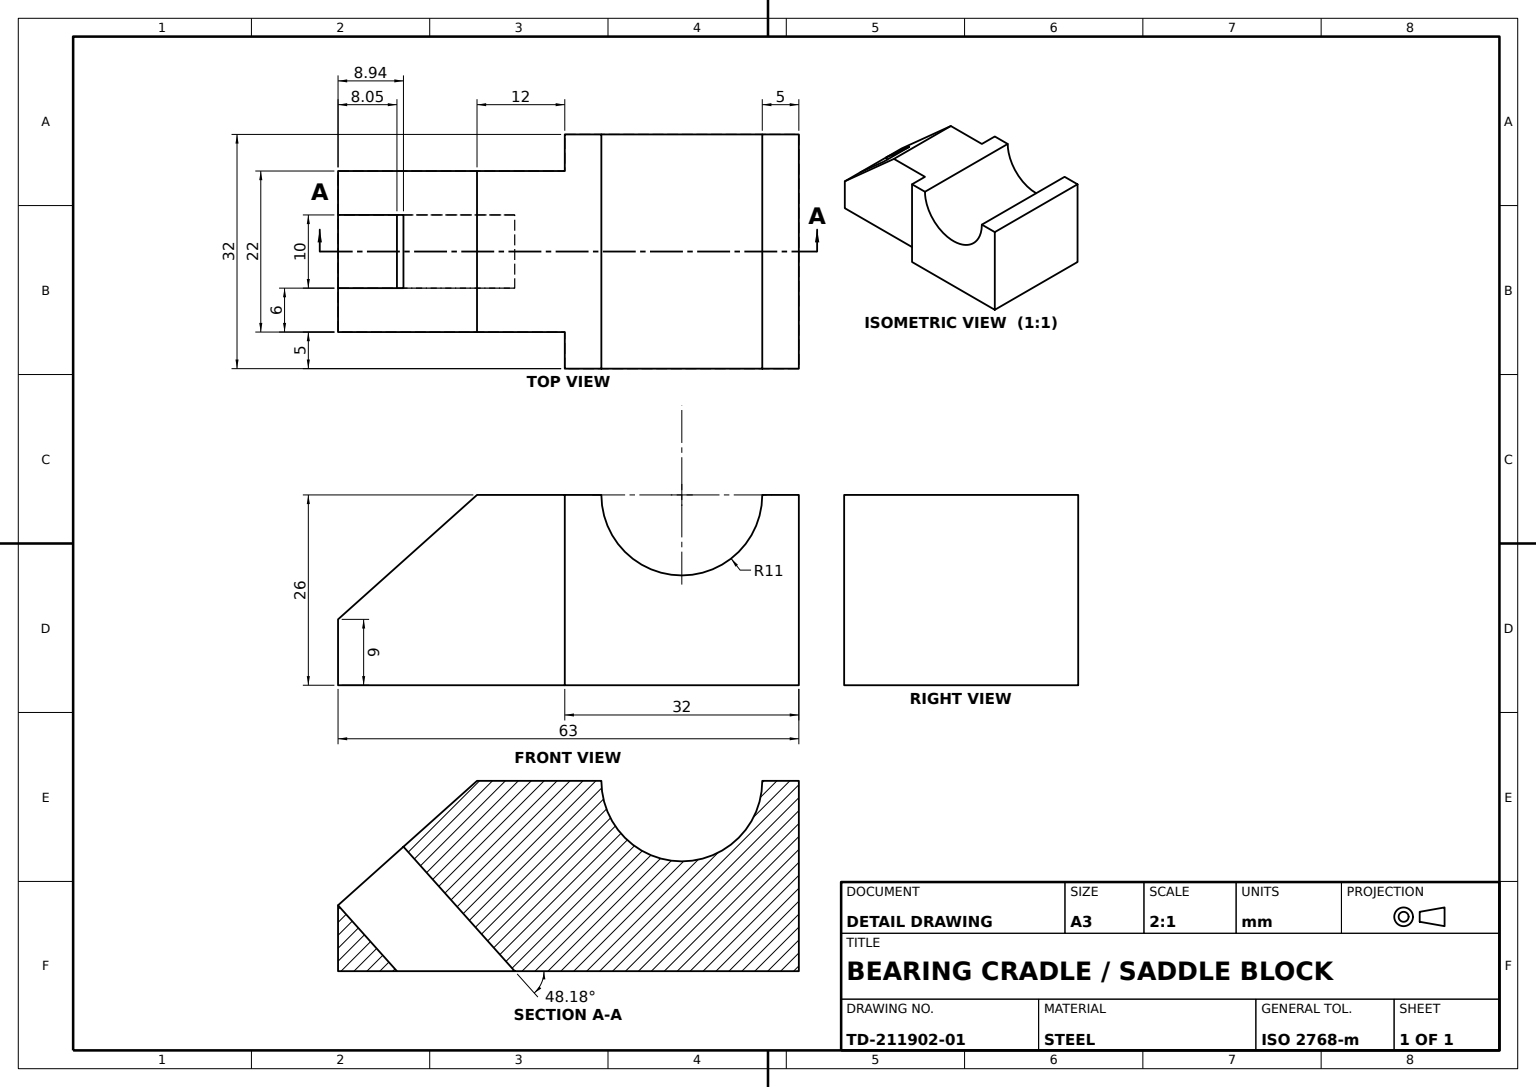
SolidWorks part; units mm, degrees
material "Plain Carbon Steel"
ref_plane "Front Plane" through (0, 0, 0) normal (0, 0, 1) x (1, 0, 0)
ref_plane "Top Plane" through (0, 0, 0) normal (0, 1, 0) x (1, 0, 0)
ref_plane "Right Plane" through (0, 0, 0) normal (1, 0, 0) x (0, 0, -1)
sketch "Cradle Block Profile" plane through (0, 0, 0) normal (0, 0, 1) x (1, 0, 0)
  line L0 (11, 13) -> (16, 13)
  line L5 (-16, 13) -> (-11, 13)
  line L6 (-16, 13) -> (-16, -13)
  line L11 (-16, -13) -> (16, -13)
  line L12 (16, 13) -> (16, -13)
  line L13 (-16, 13) -> (16, -13) construction
  line L14 (-16, -13) -> (16, 13) construction
  arc A0 (-11, 13) -> (11, 13) centre (0, 13) ccw
  point P0 (0, 0)
  dimension "D3" = 11
  dimension "D1" = 32
  dimension "D2" = 26
  dimension "D4" = 16
  dimension "D5" = 5
extrude "Cradle Block" add sketch "Cradle Block Profile" along normal mid plane 32
sketch "Tapered Extension Profile" plane through (0, 0, 0) normal (0, 0, 1) x (1, 0, 0)
  line L0 (-16, 13) -> (-28, 13)
  line L1 (-28, 13) -> (-47, -4)
  line L2 (-47, -4) -> (-47, -13)
  line L3 (-47, -13) -> (-16, -13)
  line L4 (-16, 13) -> (-16, -13)
  dimension "D1" = 9
  dimension "D2" = 12
  dimension "D3" = 63
extrude "Tapered Extension" add sketch "Tapered Extension Profile" along normal mid plane 22
sketch "Relief Slot Profile" plane through (-18.9092, 21.1338, 0) normal (-0.6668, 0.7452, 0) x (0.7452, 0.6668, 0)
  line L0 (-37.6935, 5) -> (-25.6935, 5)
  line L1 (-37.6935, -11) -> (-37.6935, 11) construction
  line L2 (-25.6935, 5) -> (-25.6935, -5)
  line L3 (-25.6935, -5) -> (-37.6935, -5)
  line L6 (-37.6935, 5) -> (-37.6935, -5)
  dimension "D1" = 10
  dimension "D2" = 12
  dimension "D3" = 6
extrude "Relief Slot" cut sketch "Relief Slot Profile" against normal through all
